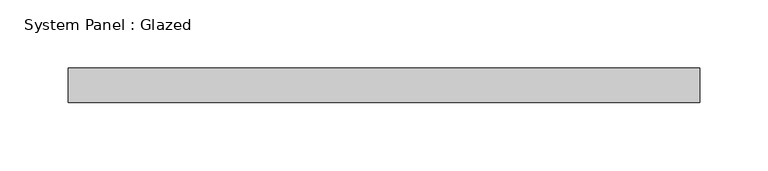
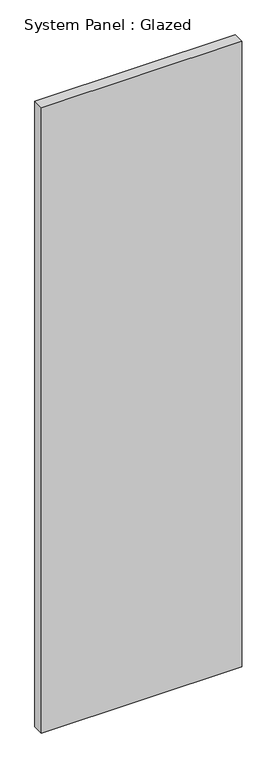
"""IFC4 building model written with IfcOpenShell, lengths in millimetres: plate geometry, System Panel : Glazed."""

from ifc_helpers import new_model, si_unit, origin, origin_with_axes, place, context, project, spatial, polyline, outline, extrude, source, transform, mapped, element, save


def system_panel_glazed_c29ca9bc(model_context):
    return source(origin(), model_context, "Body", "SweptSolid", [
        extrude(outline(polyline([(231.775, 19.05), (-231.775, 19.05), (-231.775, 44.45), (231.775, 44.45), (231.775, 19.05)])), origin_with_axes(), (0.0, 0.0, 1.0), 1529.4112238),
    ])


if __name__ == "__main__":
    model = new_model("IFC4")
    model_context = context("Model", 3, world=origin())
    ifc_project = project(units=[si_unit("LENGTHUNIT", "METRE", prefix="MILLI")], contexts=[model_context])
    site = spatial("IfcSite", under=ifc_project)
    building = spatial("IfcBuilding", under=site)
    placement = place(None, origin())
    system_panel_glazed_shape = system_panel_glazed_c29ca9bc(model_context)
    element("IfcPlate", 1, ObjectType="System Panel : Glazed", at=placement, inside=building, context=model_context, shape_type="MappedRepresentation", body=[
        mapped(system_panel_glazed_shape, transform((0.0, 0.0, 0.0), x_axis=(1.0, 0.0, 0.0), y_axis=(0.0, 1.0, 0.0), z_axis=(0.0, 0.0, 1.0))),
    ])
    save(model, "model.ifc")

# Revit data of these elements
# Type "System Panel : Glazed"
#   Construction Type Id = "GSP4R"
#   Analytic Construction = "1/8 in Pilkington single glazing"
#   Visual Light Transmittance = 0.9
#   Solar Heat Gain Coefficient = 0.86
#   Heat Transfer Coefficient (U) = 1.18115 BTU/(h·ft²·°F)
#   Define Thermal Properties by = 1
# Element 1 (IfcPlate, "System Panel : Glazed")
#   Materials on its faces: "Glass"
# Materials
#   "Glass": class "Glass", colour RGB 0 128 192, transparency 0.75, Description = "Soda Lime Glass", Cost = 0
